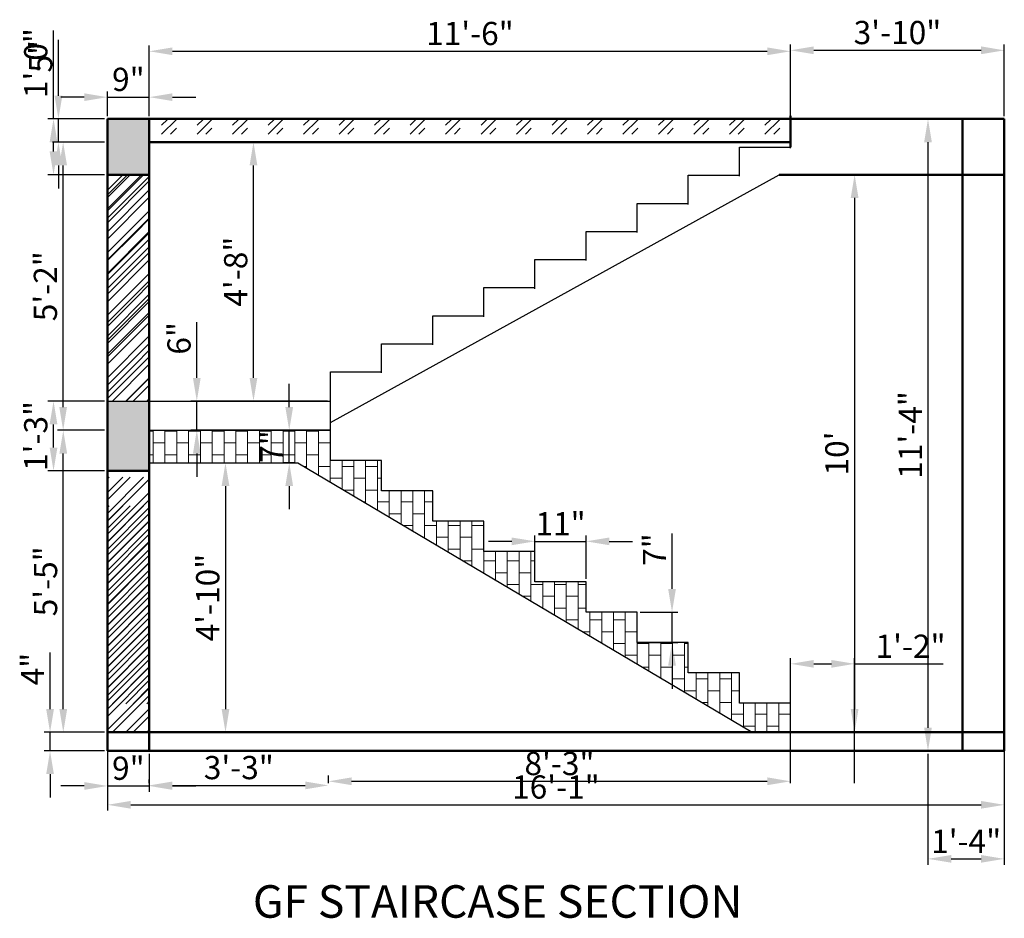
# Model space of a CAD drawing. Units: inches. Extents: x 1925 to 2200, y 918 to 1361.
# Tile 2 of 2: x 1955 to 2167, y 1168 to 1361. Entities that reach past the tile are written whole.
import ezdxf

# ---------------------------------------------------------------- set-up
doc = ezdxf.new("R2010")
doc.units = ezdxf.units.IN
for name, color, linetype, lineweight in [('A-ANNO-DIMS', 2, 'Continuous', 18), ('A-ANNO-TEXT', 7, 'Continuous', 25), ('A-FLOR-STRS', 4, 'Continuous', 25), ('A-SECT', 7, 'Continuous', 50), ('A-WALL-PATT', 8, 'Continuous', 13), ('S-COLS-PATT', 1, 'Continuous', 13), ('S-SLAB-PATT', 252, 'Continuous', 13)]:
    doc.layers.add(name, color=color, linetype=linetype, lineweight=lineweight)
doc.styles.get("Standard").update_dxf_attribs({"font": 'arial.ttf'})
doc.dimstyles.new('ISO-25', dxfattribs={"dimtxt": 5, "dimasz": 5, "dimexe": 1.25, "dimexo": 0.625, "dimtad": 1, "dimdec": 0, "dimlunit": 3, "dimtxsty": 'Standard', "dimcen": 2.5, "dimadec": 0, "dimazin": 0, "dimtfac": 1, "dimtdec": 0, "dimtmove": 0, "dimatfit": 3, "dimfxl": 1, "dimarcsym": 0})

# ---------------------------------------------------------------- blocks, each defined once
blk = doc.blocks.new('*D18')
at = {"layer": 'A-ANNO-DIMS', "color": 0, "lineweight": -2, "transparency": 16777216}
for p, q in [((1961.55, 1212.71), (1961.55, 1224.91)), ((1973.27, 1207.71), (1960.3, 1207.71)), ((1961.55, 1203.71), (1961.55, 1207.71)), ((1973.27, 1203.71), (1960.3, 1203.71)), ((1961.55, 1198.71), (1961.55, 1193.71))]:
    blk.add_line(p, q, dxfattribs=at)
at = {"layer": 'A-ANNO-DIMS', "color": 0, "transparency": 16777216}
for points in [[(1960.72, 1212.71), (1962.38, 1212.71), (1961.55, 1207.71)], [(1960.72, 1198.71), (1962.38, 1198.71), (1961.55, 1203.71)]]:
    blk.add_solid(points, dxfattribs=at)
at = {"layer": 'Defpoints', "color": 0, "transparency": 16777216}
for p in [(1961.55, 1207.71), (1973.9, 1207.71), (1973.9, 1203.71)]:
    blk.add_point(p, dxfattribs=at)
at = {"layer": 'A-ANNO-DIMS', "color": 0, "transparency": 16777216, "insert": (1958.43, 1221.31), "char_height": 5, "attachment_point": 5, "rotation": 90}
blk.add_mtext('4"', dxfattribs=at)
blk = doc.blocks.new('*D19')
at = {"layer": 'A-ANNO-DIMS', "color": 0, "lineweight": -2, "transparency": 16777216}
for p, q in [((1973.27, 1272.71), (1963.15, 1272.71)), ((1964.4, 1212.71), (1964.4, 1267.71)), ((1973.27, 1207.71), (1963.15, 1207.71))]:
    blk.add_line(p, q, dxfattribs=at)
at = {"layer": 'A-ANNO-DIMS', "color": 0, "transparency": 16777216}
for points in [[(1963.56, 1267.71), (1965.23, 1267.71), (1964.4, 1272.71)], [(1963.56, 1212.71), (1965.23, 1212.71), (1964.4, 1207.71)]]:
    blk.add_solid(points, dxfattribs=at)
at = {"layer": 'Defpoints', "color": 0, "transparency": 16777216}
for p in [(1964.4, 1272.71), (1973.9, 1272.71), (1973.9, 1207.71)]:
    blk.add_point(p, dxfattribs=at)
at = {"layer": 'A-ANNO-DIMS', "color": 0, "transparency": 16777216, "insert": (1961.23, 1240.21), "char_height": 5, "attachment_point": 5, "rotation": 90}
blk.add_mtext('5\'-5"', dxfattribs=at)
blk = doc.blocks.new('*D20')
at = {"layer": 'A-ANNO-DIMS', "color": 0, "lineweight": -2, "transparency": 16777216}
for p, q in [((1973.27, 1334.71), (1963.12, 1334.71)), ((1964.37, 1277.71), (1964.37, 1329.71)), ((1973.27, 1272.71), (1963.12, 1272.71))]:
    blk.add_line(p, q, dxfattribs=at)
at = {"layer": 'A-ANNO-DIMS', "color": 0, "transparency": 16777216}
for points in [[(1963.54, 1329.71), (1965.2, 1329.71), (1964.37, 1334.71)], [(1963.54, 1277.71), (1965.2, 1277.71), (1964.37, 1272.71)]]:
    blk.add_solid(points, dxfattribs=at)
at = {"layer": 'Defpoints', "color": 0, "transparency": 16777216}
for p in [(1964.37, 1334.71), (1973.9, 1334.71), (1973.9, 1272.71)]:
    blk.add_point(p, dxfattribs=at)
at = {"layer": 'A-ANNO-DIMS', "color": 0, "transparency": 16777216, "insert": (1961.19, 1303.71), "char_height": 5, "attachment_point": 5, "rotation": 90}
blk.add_mtext('5\'-2"', dxfattribs=at)
blk = doc.blocks.new('*D21')
at = {"layer": 'A-ANNO-DIMS', "color": 0, "lineweight": -2, "transparency": 16777216}
for p, q in [((1963.35, 1344.71), (1963.35, 1356.71)), ((1973.27, 1339.71), (1962.1, 1339.71)), ((1963.35, 1334.71), (1963.35, 1339.71)), ((1973.27, 1334.71), (1962.1, 1334.71)), ((1963.35, 1329.71), (1963.35, 1324.71))]:
    blk.add_line(p, q, dxfattribs=at)
at = {"layer": 'A-ANNO-DIMS', "color": 0, "transparency": 16777216}
for points in [[(1962.52, 1344.71), (1964.19, 1344.71), (1963.35, 1339.71)], [(1962.52, 1329.71), (1964.19, 1329.71), (1963.35, 1334.71)]]:
    blk.add_solid(points, dxfattribs=at)
at = {"layer": 'Defpoints', "color": 0, "transparency": 16777216}
for p in [(1963.35, 1339.71), (1973.9, 1339.71), (1973.9, 1334.71)]:
    blk.add_point(p, dxfattribs=at)
at = {"layer": 'A-ANNO-DIMS', "color": 0, "transparency": 16777216, "insert": (1960.18, 1353.21), "char_height": 5, "attachment_point": 5, "rotation": 90}
blk.add_mtext('5"', dxfattribs=at)
blk = doc.blocks.new('*D22')
at = {"layer": 'A-ANNO-DIMS', "color": 0, "lineweight": -2, "transparency": 16777216}
for p, q in [((1999.5, 1265.71), (2000.55, 1265.71)), ((1999.3, 1260.71), (1999.3, 1212.71)), ((1999.5, 1207.71), (2000.55, 1207.71))]:
    blk.add_line(p, q, dxfattribs=at)
at = {"layer": 'A-ANNO-DIMS', "color": 0, "transparency": 16777216}
for points in [[(1998.47, 1260.71), (2000.14, 1260.71), (1999.3, 1265.71)], [(1998.47, 1212.71), (2000.14, 1212.71), (1999.3, 1207.71)]]:
    blk.add_solid(points, dxfattribs=at)
at = {"layer": 'Defpoints', "color": 0, "transparency": 16777216}
for p in [(1998.87, 1265.71), (1998.87, 1207.71), (1999.3, 1207.71)]:
    blk.add_point(p, dxfattribs=at)
at = {"layer": 'A-ANNO-DIMS', "color": 0, "transparency": 16777216, "insert": (1996.13, 1236.71), "char_height": 5, "attachment_point": 5, "rotation": 90}
blk.add_mtext('4\'-10"', dxfattribs=at)
blk = doc.blocks.new('*D23')
at = {"layer": 'A-ANNO-DIMS', "color": 0, "lineweight": -2, "transparency": 16777216}
for p, q in [((1999.93, 1334.71), (2006.58, 1334.71)), ((2005.33, 1283.99), (2005.33, 1329.71)), ((1999.93, 1278.99), (2006.58, 1278.99))]:
    blk.add_line(p, q, dxfattribs=at)
at = {"layer": 'A-ANNO-DIMS', "color": 0, "transparency": 16777216}
for points in [[(2004.49, 1329.71), (2006.16, 1329.71), (2005.33, 1334.71)], [(2004.49, 1283.99), (2006.16, 1283.99), (2005.33, 1278.99)]]:
    blk.add_solid(points, dxfattribs=at)
at = {"layer": 'Defpoints', "color": 0, "transparency": 16777216}
for p in [(1999.3, 1334.71), (2005.33, 1334.71), (1999.3, 1278.99)]:
    blk.add_point(p, dxfattribs=at)
at = {"layer": 'A-ANNO-DIMS', "color": 0, "transparency": 16777216, "insert": (2002.15, 1306.85), "char_height": 5, "attachment_point": 5, "rotation": 90}
blk.add_mtext('4\'-8"', dxfattribs=at)
blk = doc.blocks.new('*D24')
at = {"layer": 'A-ANNO-DIMS', "color": 0, "lineweight": -2, "transparency": 16777216}
for p, q in [((1973.9, 1340.33), (1973.9, 1345.65)), ((1982.9, 1340.33), (1982.9, 1345.65)), ((1968.9, 1344.4), (1963.9, 1344.4)), ((1973.9, 1344.4), (1982.9, 1344.4)), ((1987.9, 1344.4), (1992.9, 1344.4))]:
    blk.add_line(p, q, dxfattribs=at)
at = {"layer": 'A-ANNO-DIMS', "color": 0, "transparency": 16777216}
for points in [[(1968.9, 1345.23), (1968.9, 1343.57), (1973.9, 1344.4)], [(1987.9, 1345.23), (1987.9, 1343.57), (1982.9, 1344.4)]]:
    blk.add_solid(points, dxfattribs=at)
at = {"layer": 'Defpoints', "color": 0, "transparency": 16777216}
for p in [(1982.9, 1344.4), (1973.9, 1339.71), (1982.9, 1339.71)]:
    blk.add_point(p, dxfattribs=at)
at = {"layer": 'A-ANNO-DIMS', "color": 0, "transparency": 16777216, "insert": (1978.4, 1347.58), "char_height": 5, "attachment_point": 5}
blk.add_mtext('9"', dxfattribs=at)
blk = doc.blocks.new('*D25')
at = {"layer": 'A-ANNO-DIMS', "color": 0, "lineweight": -2, "transparency": 16777216}
for p, q in [((1982.9, 1340.33), (1982.9, 1355.52)), ((1987.9, 1354.27), (2115.9, 1354.27)), ((2120.9, 1341.01), (2120.9, 1355.52))]:
    blk.add_line(p, q, dxfattribs=at)
at = {"layer": 'A-ANNO-DIMS', "color": 0, "transparency": 16777216}
for points in [[(1987.9, 1355.1), (1987.9, 1353.44), (1982.9, 1354.27)], [(2115.9, 1355.1), (2115.9, 1353.44), (2120.9, 1354.27)]]:
    blk.add_solid(points, dxfattribs=at)
at = {"layer": 'Defpoints', "color": 0, "transparency": 16777216}
for p in [(2120.9, 1354.27), (1982.9, 1339.71), (2120.9, 1340.38)]:
    blk.add_point(p, dxfattribs=at)
at = {"layer": 'A-ANNO-DIMS', "color": 0, "transparency": 16777216, "insert": (2051.9, 1357.45), "char_height": 5, "attachment_point": 5}
blk.add_mtext('11\'-6"', dxfattribs=at)
blk = doc.blocks.new('*D26')
at = {"layer": 'A-ANNO-DIMS', "color": 0, "lineweight": -2, "transparency": 16777216}
for p, q in [((2120.9, 1340.32), (2120.9, 1355.73)), ((2125.9, 1354.48), (2161.9, 1354.48)), ((2166.9, 1340.32), (2166.9, 1355.73))]:
    blk.add_line(p, q, dxfattribs=at)
at = {"layer": 'A-ANNO-DIMS', "color": 0, "transparency": 16777216}
for points in [[(2125.9, 1355.32), (2125.9, 1353.65), (2120.9, 1354.48)], [(2161.9, 1355.32), (2161.9, 1353.65), (2166.9, 1354.48)]]:
    blk.add_solid(points, dxfattribs=at)
at = {"layer": 'Defpoints', "color": 0, "transparency": 16777216}
for p in [(2166.9, 1354.48), (2120.9, 1339.69), (2166.9, 1339.69)]:
    blk.add_point(p, dxfattribs=at)
at = {"layer": 'A-ANNO-DIMS', "color": 0, "transparency": 16777216, "insert": (2143.9, 1357.66), "char_height": 5, "attachment_point": 5}
blk.add_mtext('3\'-10"', dxfattribs=at)
blk = doc.blocks.new('*D27')
at = {"layer": 'A-ANNO-DIMS', "color": 0, "lineweight": -2, "transparency": 16777216}
for p, q in [((2142.03, 1327.71), (2133.43, 1327.71)), ((2134.68, 1322.71), (2134.68, 1212.71)), ((2142.03, 1207.71), (2133.43, 1207.71))]:
    blk.add_line(p, q, dxfattribs=at)
at = {"layer": 'A-ANNO-DIMS', "color": 0, "transparency": 16777216}
for points in [[(2133.85, 1322.71), (2135.52, 1322.71), (2134.68, 1327.71)], [(2133.85, 1212.71), (2135.52, 1212.71), (2134.68, 1207.71)]]:
    blk.add_solid(points, dxfattribs=at)
at = {"layer": 'Defpoints', "color": 0, "transparency": 16777216}
for p in [(2142.66, 1327.71), (2134.68, 1207.71), (2142.66, 1207.71)]:
    blk.add_point(p, dxfattribs=at)
at = {"layer": 'A-ANNO-DIMS', "color": 0, "transparency": 16777216, "insert": (2131.51, 1267.71), "char_height": 5, "attachment_point": 5, "rotation": 90}
blk.add_mtext("10'", dxfattribs=at)
blk = doc.blocks.new('*D28')
at = {"layer": 'A-ANNO-DIMS', "color": 0, "lineweight": -2, "transparency": 16777216}
for p, q in [((2157.27, 1339.71), (2149.22, 1339.71)), ((2150.47, 1334.71), (2150.47, 1208.71)), ((2157.27, 1203.71), (2149.22, 1203.71))]:
    blk.add_line(p, q, dxfattribs=at)
at = {"layer": 'A-ANNO-DIMS', "color": 0, "transparency": 16777216}
for points in [[(2149.64, 1334.71), (2151.3, 1334.71), (2150.47, 1339.71)], [(2149.64, 1208.71), (2151.3, 1208.71), (2150.47, 1203.71)]]:
    blk.add_solid(points, dxfattribs=at)
at = {"layer": 'Defpoints', "color": 0, "transparency": 16777216}
for p in [(2157.9, 1339.71), (2150.47, 1203.71), (2157.9, 1203.71)]:
    blk.add_point(p, dxfattribs=at)
at = {"layer": 'A-ANNO-DIMS', "color": 0, "transparency": 16777216, "insert": (2147.33, 1271.71), "char_height": 5, "attachment_point": 5, "rotation": 90}
blk.add_mtext('11\'-4"', dxfattribs=at)
blk = doc.blocks.new('*D29')
at = {"layer": 'A-ANNO-DIMS', "color": 0, "lineweight": -2, "transparency": 16777216}
for p, q in [((1973.9, 1203.08), (1973.9, 1194.92)), ((1982.9, 1203.08), (1982.9, 1194.92)), ((1968.9, 1196.17), (1963.9, 1196.17)), ((1973.9, 1196.17), (1982.9, 1196.17)), ((1987.9, 1196.17), (1992.9, 1196.17))]:
    blk.add_line(p, q, dxfattribs=at)
at = {"layer": 'A-ANNO-DIMS', "color": 0, "transparency": 16777216}
for points in [[(1968.9, 1197), (1968.9, 1195.33), (1973.9, 1196.17)], [(1987.9, 1197), (1987.9, 1195.33), (1982.9, 1196.17)]]:
    blk.add_solid(points, dxfattribs=at)
at = {"layer": 'Defpoints', "color": 0, "transparency": 16777216}
for p in [(1973.9, 1203.71), (1982.9, 1203.71), (1982.9, 1196.17)]:
    blk.add_point(p, dxfattribs=at)
at = {"layer": 'A-ANNO-DIMS', "color": 0, "transparency": 16777216, "insert": (1978.4, 1199.34), "char_height": 5, "attachment_point": 5}
blk.add_mtext('9"', dxfattribs=at)
blk = doc.blocks.new('*D30')
at = {"layer": 'A-ANNO-DIMS', "color": 0, "lineweight": -2, "transparency": 16777216}
for p, q in [((1982.9, 1196.79), (1982.9, 1197.54)), ((2021.45, 1196.79), (2021.45, 1197.54)), ((1987.9, 1196.29), (2016.45, 1196.29))]:
    blk.add_line(p, q, dxfattribs=at)
at = {"layer": 'A-ANNO-DIMS', "color": 0, "transparency": 16777216}
for points in [[(1987.9, 1197.12), (1987.9, 1195.45), (1982.9, 1196.29)], [(2016.45, 1197.12), (2016.45, 1195.45), (2021.45, 1196.29)]]:
    blk.add_solid(points, dxfattribs=at)
at = {"layer": 'Defpoints', "color": 0, "transparency": 16777216}
for p in [(1982.9, 1196.17), (2021.45, 1196.29), (2021.45, 1196.17)]:
    blk.add_point(p, dxfattribs=at)
at = {"layer": 'A-ANNO-DIMS', "color": 0, "transparency": 16777216, "insert": (2002.17, 1199.47), "char_height": 5, "attachment_point": 5}
blk.add_mtext('3\'-3"', dxfattribs=at)
blk = doc.blocks.new('*D31')
at = {"layer": 'A-ANNO-DIMS', "color": 0, "lineweight": -2, "transparency": 16777216}
for p, q in [((2021.45, 1196.79), (2021.45, 1198.42)), ((2026.45, 1197.17), (2115.9, 1197.17)), ((2120.9, 1196.79), (2120.9, 1198.42))]:
    blk.add_line(p, q, dxfattribs=at)
at = {"layer": 'A-ANNO-DIMS', "color": 0, "transparency": 16777216}
for points in [[(2026.45, 1198.01), (2026.45, 1196.34), (2021.45, 1197.17)], [(2115.9, 1198.01), (2115.9, 1196.34), (2120.9, 1197.17)]]:
    blk.add_solid(points, dxfattribs=at)
at = {"layer": 'Defpoints', "color": 0, "transparency": 16777216}
for p in [(2120.9, 1197.17), (2021.45, 1196.17), (2120.9, 1196.17)]:
    blk.add_point(p, dxfattribs=at)
at = {"layer": 'A-ANNO-DIMS', "color": 0, "transparency": 16777216, "insert": (2071.17, 1200.35), "char_height": 5, "attachment_point": 5}
blk.add_mtext('8\'-3"', dxfattribs=at)
blk = doc.blocks.new('*D32')
at = {"layer": 'A-ANNO-DIMS', "color": 0, "lineweight": -2, "transparency": 16777216}
for p, q in [((2120.9, 1196.79), (2120.9, 1223.7)), ((2134.68, 1196.79), (2134.68, 1223.7)), ((2125.9, 1222.45), (2129.68, 1222.45)), ((2134.68, 1222.45), (2153.75, 1222.45))]:
    blk.add_line(p, q, dxfattribs=at)
at = {"layer": 'A-ANNO-DIMS', "color": 0, "transparency": 16777216}
for points in [[(2125.9, 1223.28), (2125.9, 1221.62), (2120.9, 1222.45)], [(2129.68, 1223.28), (2129.68, 1221.62), (2134.68, 1222.45)]]:
    blk.add_solid(points, dxfattribs=at)
at = {"layer": 'Defpoints', "color": 0, "transparency": 16777216}
for p in [(2134.68, 1222.45), (2120.9, 1196.17), (2134.68, 1196.17)]:
    blk.add_point(p, dxfattribs=at)
at = {"layer": 'A-ANNO-DIMS', "color": 0, "transparency": 16777216, "insert": (2146.72, 1225.59), "char_height": 5, "attachment_point": 5}
blk.add_mtext('1\'-2"', dxfattribs=at)
blk = doc.blocks.new('*D33')
at = {"layer": 'A-ANNO-DIMS', "color": 0, "lineweight": -2, "transparency": 16777216}
for p, q in [((2150.47, 1203.08), (2150.47, 1179.23)), ((2166.9, 1203.08), (2166.9, 1179.23)), ((2155.47, 1180.48), (2161.9, 1180.48))]:
    blk.add_line(p, q, dxfattribs=at)
at = {"layer": 'A-ANNO-DIMS', "color": 0, "transparency": 16777216}
for points in [[(2155.47, 1181.31), (2155.47, 1179.65), (2150.47, 1180.48)], [(2161.9, 1181.31), (2161.9, 1179.65), (2166.9, 1180.48)]]:
    blk.add_solid(points, dxfattribs=at)
at = {"layer": 'Defpoints', "color": 0, "transparency": 16777216}
for p in [(2150.47, 1203.71), (2166.9, 1203.71), (2166.9, 1180.48)]:
    blk.add_point(p, dxfattribs=at)
at = {"layer": 'A-ANNO-DIMS', "color": 0, "transparency": 16777216, "insert": (2158.68, 1183.61), "char_height": 5, "attachment_point": 5}
blk.add_mtext('1\'-4"', dxfattribs=at)
blk = doc.blocks.new('*D34')
at = {"layer": 'A-ANNO-DIMS', "color": 0, "lineweight": -2, "transparency": 16777216}
for p, q in [((2060.9, 1248.81), (2055.9, 1248.81)), ((2065.9, 1240.71), (2065.9, 1250.06)), ((2065.9, 1248.81), (2076.9, 1248.81)), ((2076.9, 1240.71), (2076.9, 1250.06)), ((2081.9, 1248.81), (2086.9, 1248.81))]:
    blk.add_line(p, q, dxfattribs=at)
at = {"layer": 'A-ANNO-DIMS', "color": 0, "transparency": 16777216}
for points in [[(2060.9, 1249.64), (2060.9, 1247.98), (2065.9, 1248.81)], [(2081.9, 1249.64), (2081.9, 1247.98), (2076.9, 1248.81)]]:
    blk.add_solid(points, dxfattribs=at)
at = {"layer": 'Defpoints', "color": 0, "transparency": 16777216}
for p in [(2076.9, 1248.81), (2065.9, 1240.09), (2076.9, 1240.09)]:
    blk.add_point(p, dxfattribs=at)
at = {"layer": 'A-ANNO-DIMS', "color": 0, "transparency": 16777216, "insert": (2071.4, 1251.95), "char_height": 5, "attachment_point": 5}
blk.add_mtext('11"', dxfattribs=at)
blk = doc.blocks.new('*D35')
at = {"layer": 'A-ANNO-DIMS', "color": 0, "lineweight": -2, "transparency": 16777216}
for p, q in [((2095.39, 1238.56), (2095.39, 1250.52)), ((2088.52, 1233.56), (2096.64, 1233.56)), ((2095.39, 1227.04), (2095.39, 1233.56)), ((2088.52, 1227.04), (2096.64, 1227.04)), ((2095.39, 1222.04), (2095.39, 1217.04))]:
    blk.add_line(p, q, dxfattribs=at)
at = {"layer": 'A-ANNO-DIMS', "color": 0, "transparency": 16777216}
for points in [[(2094.56, 1238.56), (2096.23, 1238.56), (2095.39, 1233.56)], [(2094.56, 1222.04), (2096.23, 1222.04), (2095.39, 1227.04)]]:
    blk.add_solid(points, dxfattribs=at)
at = {"layer": 'Defpoints', "color": 0, "transparency": 16777216}
for p in [(2087.9, 1233.56), (2095.39, 1233.56), (2087.9, 1227.04)]:
    blk.add_point(p, dxfattribs=at)
at = {"layer": 'A-ANNO-DIMS', "color": 0, "transparency": 16777216, "insert": (2092.27, 1247.04), "char_height": 5, "attachment_point": 5, "rotation": 90}
blk.add_mtext('7"', dxfattribs=at)
blk = doc.blocks.new('*D36')
at = {"layer": 'A-ANNO-DIMS', "color": 0, "lineweight": -2, "transparency": 16777216}
for p, q in [((2013.02, 1277.71), (2013.02, 1282.71)), ((2014.23, 1272.71), (2011.77, 1272.71)), ((2013.02, 1265.71), (2013.02, 1272.71)), ((2014.23, 1265.71), (2011.77, 1265.71)), ((2013.02, 1260.71), (2013.02, 1255.71))]:
    blk.add_line(p, q, dxfattribs=at)
at = {"layer": 'A-ANNO-DIMS', "color": 0, "transparency": 16777216}
for points in [[(2012.18, 1277.71), (2013.85, 1277.71), (2013.02, 1272.71)], [(2012.18, 1260.71), (2013.85, 1260.71), (2013.02, 1265.71)]]:
    blk.add_solid(points, dxfattribs=at)
at = {"layer": 'Defpoints', "color": 0, "transparency": 16777216}
for p in [(2013.02, 1272.71), (2014.85, 1272.71), (2014.85, 1265.71)]:
    blk.add_point(p, dxfattribs=at)
at = {"layer": 'A-ANNO-DIMS', "color": 0, "transparency": 16777216, "insert": (2009.89, 1269.21), "char_height": 5, "attachment_point": 5, "rotation": 90}
blk.add_mtext('7"', dxfattribs=at)
blk = doc.blocks.new('*D37')
at = {"layer": 'A-ANNO-DIMS', "color": 0, "lineweight": -2, "transparency": 16777216}
for p, q in [((1993.13, 1283.99), (1993.13, 1296.01)), ((2021.27, 1278.99), (1991.88, 1278.99)), ((1993.13, 1272.71), (1993.13, 1278.99)), ((2021.27, 1272.71), (1991.88, 1272.71)), ((1993.13, 1267.71), (1993.13, 1262.71))]:
    blk.add_line(p, q, dxfattribs=at)
at = {"layer": 'A-ANNO-DIMS', "color": 0, "transparency": 16777216}
for points in [[(1992.3, 1283.99), (1993.96, 1283.99), (1993.13, 1278.99)], [(1992.3, 1267.71), (1993.96, 1267.71), (1993.13, 1272.71)]]:
    blk.add_solid(points, dxfattribs=at)
at = {"layer": 'Defpoints', "color": 0, "transparency": 16777216}
for p in [(1993.13, 1278.99), (2021.9, 1278.99), (2021.9, 1272.71)]:
    blk.add_point(p, dxfattribs=at)
at = {"layer": 'A-ANNO-DIMS', "color": 0, "transparency": 16777216, "insert": (1989.95, 1292.5), "char_height": 5, "attachment_point": 5, "rotation": 90}
blk.add_mtext('6"', dxfattribs=at)
blk = doc.blocks.new('*D42')
at = {"layer": 'A-ANNO-DIMS', "color": 0, "lineweight": -2, "transparency": 16777216}
for p, q in [((1973.9, 1207.08), (1973.9, 1190.86)), ((2166.9, 1207.08), (2166.9, 1190.86)), ((1978.9, 1192.11), (2161.9, 1192.11))]:
    blk.add_line(p, q, dxfattribs=at)
at = {"layer": 'A-ANNO-DIMS', "color": 0, "transparency": 16777216}
for points in [[(1978.9, 1192.94), (1978.9, 1191.28), (1973.9, 1192.11)], [(2161.9, 1192.94), (2161.9, 1191.28), (2166.9, 1192.11)]]:
    blk.add_solid(points, dxfattribs=at)
at = {"layer": 'Defpoints', "color": 0, "transparency": 16777216}
for p in [(1973.9, 1207.71), (2166.9, 1207.71), (2166.9, 1192.11)]:
    blk.add_point(p, dxfattribs=at)
at = {"layer": 'A-ANNO-DIMS', "color": 0, "transparency": 16777216, "insert": (2070.4, 1195.29), "char_height": 5, "attachment_point": 5}
blk.add_mtext('16\'-1"', dxfattribs=at)
blk = doc.blocks.new('*D43')
at = {"layer": 'A-ANNO-DIMS', "color": 0, "lineweight": -2, "transparency": 16777216}
for p, q in [((1962.3, 1339.71), (1962.3, 1358.78)), ((1973.27, 1339.71), (1961.05, 1339.71)), ((1962.3, 1332.71), (1962.3, 1334.71)), ((1973.27, 1327.71), (1961.05, 1327.71))]:
    blk.add_line(p, q, dxfattribs=at)
at = {"layer": 'A-ANNO-DIMS', "color": 0, "transparency": 16777216}
for points in [[(1961.46, 1334.71), (1963.13, 1334.71), (1962.3, 1339.71)], [(1961.46, 1332.71), (1963.13, 1332.71), (1962.3, 1327.71)]]:
    blk.add_solid(points, dxfattribs=at)
at = {"layer": 'Defpoints', "color": 0, "transparency": 16777216}
for p in [(1962.3, 1339.71), (1973.9, 1339.71), (1973.9, 1327.71)]:
    blk.add_point(p, dxfattribs=at)
at = {"layer": 'A-ANNO-DIMS', "color": 0, "transparency": 16777216, "insert": (1959.12, 1351.74), "char_height": 5, "attachment_point": 5, "rotation": 90}
blk.add_mtext('1\'-0"', dxfattribs=at)
blk = doc.blocks.new('*D44')
at = {"layer": 'A-ANNO-DIMS', "color": 0, "lineweight": -2, "transparency": 16777216}
for p, q in [((1973.27, 1278.99), (1961.05, 1278.99)), ((1962.3, 1268.99), (1962.3, 1273.99)), ((1973.27, 1263.99), (1961.05, 1263.99))]:
    blk.add_line(p, q, dxfattribs=at)
at = {"layer": 'A-ANNO-DIMS', "color": 0, "transparency": 16777216}
for points in [[(1961.46, 1273.99), (1963.13, 1273.99), (1962.3, 1278.99)], [(1961.46, 1268.99), (1963.13, 1268.99), (1962.3, 1263.99)]]:
    blk.add_solid(points, dxfattribs=at)
at = {"layer": 'Defpoints', "color": 0, "transparency": 16777216}
for p in [(1962.3, 1278.99), (1973.9, 1278.99), (1973.9, 1263.99)]:
    blk.add_point(p, dxfattribs=at)
at = {"layer": 'A-ANNO-DIMS', "color": 0, "transparency": 16777216, "insert": (1959.12, 1271.49), "char_height": 5, "attachment_point": 5, "rotation": 90}
blk.add_mtext('1\'-3"', dxfattribs=at)

msp = doc.modelspace()

# ---------------------------------------------------------------- hatches: boundary and pattern name
at = {"layer": 'A-WALL-PATT'}
h = msp.add_hatch(dxfattribs=at)
h.set_pattern_fill('STEEL', color=256)
h.set_pattern_definition([(45, (0, 0), (-2.245064, 2.245064), []), (45, (0, 1.5875), (-2.245064, 2.245064), [])])
h.paths.add_polyline_path([(1982.9, 1327.71), (1973.9, 1327.71), (1973.9, 1278.99), (1982.9, 1278.99)])
h = msp.add_hatch(dxfattribs=at)
h.set_pattern_fill('GOST_GROUND', color=256)
h.paths.add_polyline_path([(1982.9, 1327.71), (1973.9, 1327.71), (1973.9, 1278.99), (1982.9, 1278.99)])
h = msp.add_hatch(dxfattribs=at)
h.set_pattern_fill('STEEL', color=256)
h.set_pattern_definition([(45, (-5e-13, -65.1165), (-2.245064, 2.245064), []), (45, (-5e-13, -63.529), (-2.245064, 2.245064), [])])
h.paths.add_polyline_path([(1982.9, 1262.59), (1973.9, 1262.59), (1973.9, 1213.87), (1982.9, 1213.87)])
h = msp.add_hatch(dxfattribs=at)
h.set_pattern_fill('STEEL', color=256)
h.set_pattern_definition([(45, (-5e-13, -71.28), (-2.245064, 2.245064), []), (45, (-5e-13, -69.6925), (-2.245064, 2.245064), [])])
h.paths.add_polyline_path([(1982.9, 1256.43), (1973.9, 1256.43), (1973.9, 1207.71), (1982.9, 1207.71)])
at = {"layer": 'S-COLS-PATT'}
h = msp.add_hatch(color=256, dxfattribs=at)
h.dxf.hatch_style = 1
h.paths.add_polyline_path([(1982.9, 1339.71), (1973.9, 1339.71), (1973.9, 1327.71), (1982.9, 1327.71)])
h = msp.add_hatch(color=256, dxfattribs=at)
h.dxf.hatch_style = 1
h.paths.add_polyline_path([(1982.9, 1278.99), (1973.9, 1278.99), (1973.9, 1263.99), (1982.9, 1263.99)])
at = {"layer": 'S-SLAB-PATT'}
h = msp.add_hatch(dxfattribs=at)
h.set_pattern_fill('GOST_GLASS', color=256, scale=0.9)
h.paths.add_polyline_path([(2120.9, 1339.71), (1982.9, 1339.71), (1982.9, 1334.71), (2120.9, 1334.71)])
h = msp.add_hatch(dxfattribs=at)
h.set_pattern_fill('BRICK', color=256, scale=0.4, angle=90)
h.paths.add_polyline_path([(2065.9, 1246.61), (2054.9, 1246.61), (2054.9, 1253.13), (2043.9, 1253.13), (2043.9, 1259.66), (2032.9, 1259.66), (2032.9, 1266.18), (2021.9, 1266.18), (2021.9, 1272.71), (2010.9, 1272.71), (1982.9, 1272.71), (1982.9, 1265.71), (2014.85, 1265.71), (2112.64, 1207.71), (2120.9, 1207.71), (2120.9, 1213.99), (2109.9, 1213.99), (2109.9, 1220.51), (2098.9, 1220.51), (2098.9, 1227.04), (2087.9, 1227.04), (2087.9, 1233.56), (2076.9, 1233.56), (2076.9, 1240.09), (2065.9, 1240.09)])
h.paths.add_polyline_path([(2015.12, 1264.78), (2015.12, 1273.64), (2004.82, 1273.64), (2004.82, 1264.78)], flags=9)

# ---------------------------------------------------------------- linework, layer by layer
at = {"layer": 'A-FLOR-STRS'}
for p, q in [((2120.9, 1333.41), (2120.9, 1339.69)), ((2120.9, 1339.69), (2131.9, 1339.69)), ((2109.9, 1327.37), (2109.9, 1333.65)), ((2109.9, 1333.65), (2120.9, 1333.65)), ((2021.9, 1274.42), (2118.42, 1327.71)), ((2098.9, 1321.32), (2098.9, 1327.6)), ((2098.9, 1327.6), (2109.9, 1327.6)), ((2087.9, 1315.27), (2087.9, 1321.55)), ((2087.9, 1321.55), (2098.9, 1321.55)), ((2076.9, 1309.23), (2076.9, 1315.51)), ((2076.9, 1315.51), (2087.9, 1315.51)), ((2065.9, 1303.18), (2065.9, 1309.46)), ((2065.9, 1309.46), (2076.9, 1309.46)), ((2054.9, 1297.13), (2054.9, 1303.41)), ((2054.9, 1303.41), (2065.9, 1303.41)), ((2043.9, 1291.08), (2043.9, 1297.36)), ((2043.9, 1297.36), (2054.9, 1297.36)), ((2032.9, 1285.04), (2032.9, 1291.32)), ((2032.9, 1291.32), (2043.9, 1291.32)), ((2021.9, 1278.99), (2021.9, 1285.27)), ((2021.9, 1285.27), (2032.9, 1285.27)), ((1973.9, 1278.99), (2021.9, 1278.99)), ((2021.9, 1272.71), (2021.9, 1278.99)), ((1982.9, 1272.71), (2021.9, 1272.71)), ((2021.9, 1272.71), (2010.9, 1272.71)), ((2021.9, 1266.18), (2021.9, 1272.71)), ((2021.9, 1266.43), (2021.9, 1272.71)), ((1982.9, 1265.71), (2014.85, 1265.71)), ((2014.85, 1265.71), (2112.64, 1207.71)), ((2032.9, 1266.18), (2021.9, 1266.18)), ((2032.9, 1259.66), (2032.9, 1266.18)), ((2043.9, 1259.66), (2032.9, 1259.66)), ((2043.9, 1253.13), (2043.9, 1259.66)), ((2054.9, 1253.13), (2043.9, 1253.13)), ((2054.9, 1246.61), (2054.9, 1253.13)), ((2065.9, 1246.61), (2054.9, 1246.61)), ((2065.9, 1240.09), (2065.9, 1246.61)), ((2076.9, 1240.09), (2065.9, 1240.09)), ((2076.9, 1233.56), (2076.9, 1240.09)), ((2087.9, 1233.56), (2076.9, 1233.56)), ((2087.9, 1227.04), (2087.9, 1233.56)), ((2098.9, 1227.04), (2087.9, 1227.04)), ((2098.9, 1220.51), (2098.9, 1227.04)), ((2109.9, 1220.51), (2098.9, 1220.51)), ((2109.9, 1213.99), (2109.9, 1220.51)), ((2120.9, 1213.99), (2109.9, 1213.99)), ((2120.9, 1207.71), (2120.9, 1213.99))]:
    msp.add_line(p, q, dxfattribs=at)
at = {"layer": 'A-SECT'}
for p, q in [((1973.9, 1203.71), (1973.9, 1339.71)), ((1973.9, 1339.71), (2166.9, 1339.71)), ((1982.9, 1203.71), (1982.9, 1339.71)), ((2120.9, 1333.65), (2120.9, 1340.38)), ((2157.9, 1203.71), (2157.9, 1339.71)), ((2166.9, 1203.71), (2166.9, 1339.71)), ((2166.9, 1334.71), (2166.9, 1339.71)), ((1982.9, 1334.71), (2120.9, 1334.71)), ((1973.9, 1327.71), (1982.9, 1327.71)), ((2118.42, 1327.71), (2166.9, 1327.71)), ((1973.9, 1263.99), (1982.9, 1263.99)), ((1973.9, 1207.71), (2166.9, 1207.71)), ((1973.9, 1203.71), (2166.9, 1203.71))]:
    msp.add_line(p, q, dxfattribs=at)

# ---------------------------------------------------------------- texts
at = {"layer": 'A-ANNO-TEXT', "insert": (2005.2, 1174.81), "char_height": 7, "attachment_point": 1}
msp.add_mtext_dynamic_manual_height_columns('{\\fArial|b1|i0|c0|p34;GF STAIRCASE SECTION}', width=329.4378, gutter_width=12.5, heights=[0], dxfattribs=at)

# ---------------------------------------------------------------- dimensions: what is measured, and where the dimension line sits
at = {"layer": 'A-ANNO-DIMS'}
for base, p1, p2, override, picture, middle in [((2120.9, 1354.27), (1982.9, 1339.71), (2120.9, 1340.38), {"dimclrd": 0, "dimclre": 0, "dimclrt": 0}, '*D25', (2051.9, 1357.45)), ((2166.9, 1354.48), (2120.9, 1339.69), (2166.9, 1339.69), {"dimclrd": 0, "dimclre": 0, "dimclrt": 0}, '*D26', (2143.9, 1357.66)), ((1982.9, 1344.4), (1973.9, 1339.71), (1982.9, 1339.71), {"dimclrd": 0, "dimclre": 0, "dimclrt": 0}, '*D24', (1978.4, 1347.58)), ((2076.9, 1248.81), (2065.9, 1240.09), (2076.9, 1240.09), {"dimclrd": 0, "dimclre": 0, "dimclrt": 0}, '*D34', (2071.4, 1251.95)), ((2134.68, 1222.45), (2120.9, 1196.17), (2134.68, 1196.17), {"dimclrd": 0, "dimclre": 0, "dimclrt": 0}, '*D32', (2146.72, 1225.59)), ((2166.9, 1192.11), (1973.9, 1207.71), (2166.9, 1207.71), {"dimdec": 1, "dimlfac": 1, "dimrnd": 0, "dimzin": 1, "dimdsep": 46, "dimlunit": 4, "dimfrac": 2}, '*D42', (2070.4, 1195.29)), ((1982.9, 1196.17), (1973.9, 1203.71), (1982.9, 1203.71), {"dimclrd": 0, "dimclre": 0, "dimclrt": 0}, '*D29', (1978.4, 1199.34)), ((2120.9, 1197.17), (2021.45, 1196.17), (2120.9, 1196.17), {"dimclrd": 0, "dimclre": 0, "dimclrt": 0}, '*D31', (2071.17, 1200.35)), ((2166.9, 1180.48), (2150.47, 1203.71), (2166.9, 1203.71), {"dimclrd": 0, "dimclre": 0, "dimclrt": 0}, '*D33', (2158.68, 1183.61)), ((2021.45, 1196.29), (1982.9, 1196.17), (2021.45, 1196.17), {"dimclrd": 0, "dimclre": 0, "dimclrt": 0}, '*D30', (2002.17, 1199.47))]:
    dim = msp.add_linear_dim(base=base, p1=p1, p2=p2, dimstyle='ISO-25', override=override, dxfattribs=at)
    dim.commit()
    dim.dimension.update_dxf_attribs({"geometry": picture, "text_midpoint": middle})
for base, p1, p2, override, picture, middle in [((1962.3, 1339.71), (1973.9, 1327.71), (1973.9, 1339.71), {"dimdec": 1, "dimlfac": 1, "dimrnd": 0, "dimzin": 1, "dimdsep": 46, "dimlunit": 4, "dimfrac": 2}, '*D43', (1959.12, 1351.74)), ((1963.35, 1339.71), (1973.9, 1334.71), (1973.9, 1339.71), {"dimclrd": 0, "dimclre": 0, "dimclrt": 0}, '*D21', (1960.18, 1353.21)), ((2150.47, 1203.71), (2157.9, 1339.71), (2157.9, 1203.71), {"dimclrd": 0, "dimclre": 0, "dimclrt": 0}, '*D28', (2147.33, 1271.71)), ((1964.37, 1334.71), (1973.9, 1272.71), (1973.9, 1334.71), {"dimclrd": 0, "dimclre": 0, "dimclrt": 0}, '*D20', (1961.19, 1303.71)), ((2005.33, 1334.71), (1999.3, 1278.99), (1999.3, 1334.71), {"dimclrd": 0, "dimclre": 0, "dimclrt": 0}, '*D23', (2002.15, 1306.85)), ((2134.68, 1207.71), (2142.66, 1327.71), (2142.66, 1207.71), {"dimclrd": 0, "dimclre": 0, "dimclrt": 0}, '*D27', (2131.51, 1267.71)), ((1993.13, 1278.99), (2021.9, 1272.71), (2021.9, 1278.99), {"dimclrd": 0, "dimclre": 0, "dimclrt": 0}, '*D37', (1989.95, 1292.5)), ((2013.02, 1272.71), (2014.85, 1265.71), (2014.85, 1272.71), {"dimclrd": 0, "dimclre": 0, "dimclrt": 0}, '*D36', (2009.89, 1269.21)), ((1962.3, 1278.99), (1973.9, 1263.99), (1973.9, 1278.99), {"dimdec": 1, "dimlfac": 1, "dimrnd": 0, "dimzin": 1, "dimdsep": 46, "dimlunit": 4, "dimfrac": 2}, '*D44', (1959.12, 1271.49)), ((1964.4, 1272.71), (1973.9, 1207.71), (1973.9, 1272.71), {"dimclrd": 0, "dimclre": 0, "dimclrt": 0}, '*D19', (1961.23, 1240.21)), ((1999.3, 1207.71), (1998.87, 1265.71), (1998.87, 1207.71), {"dimclrd": 0, "dimclre": 0, "dimclrt": 0}, '*D22', (1996.13, 1236.71)), ((2095.39, 1233.56), (2087.9, 1227.04), (2087.9, 1233.56), {"dimclrd": 0, "dimclre": 0, "dimclrt": 0}, '*D35', (2092.27, 1247.04)), ((1961.55, 1207.71), (1973.9, 1203.71), (1973.9, 1207.71), {"dimclrd": 0, "dimclre": 0, "dimclrt": 0}, '*D18', (1958.43, 1221.31))]:
    dim = msp.add_linear_dim(base=base, p1=p1, p2=p2, angle=90, dimstyle='ISO-25', override=override, dxfattribs=at)
    dim.commit()
    dim.dimension.update_dxf_attribs({"geometry": picture, "text_midpoint": middle})

doc.saveas('drawing.dxf')
